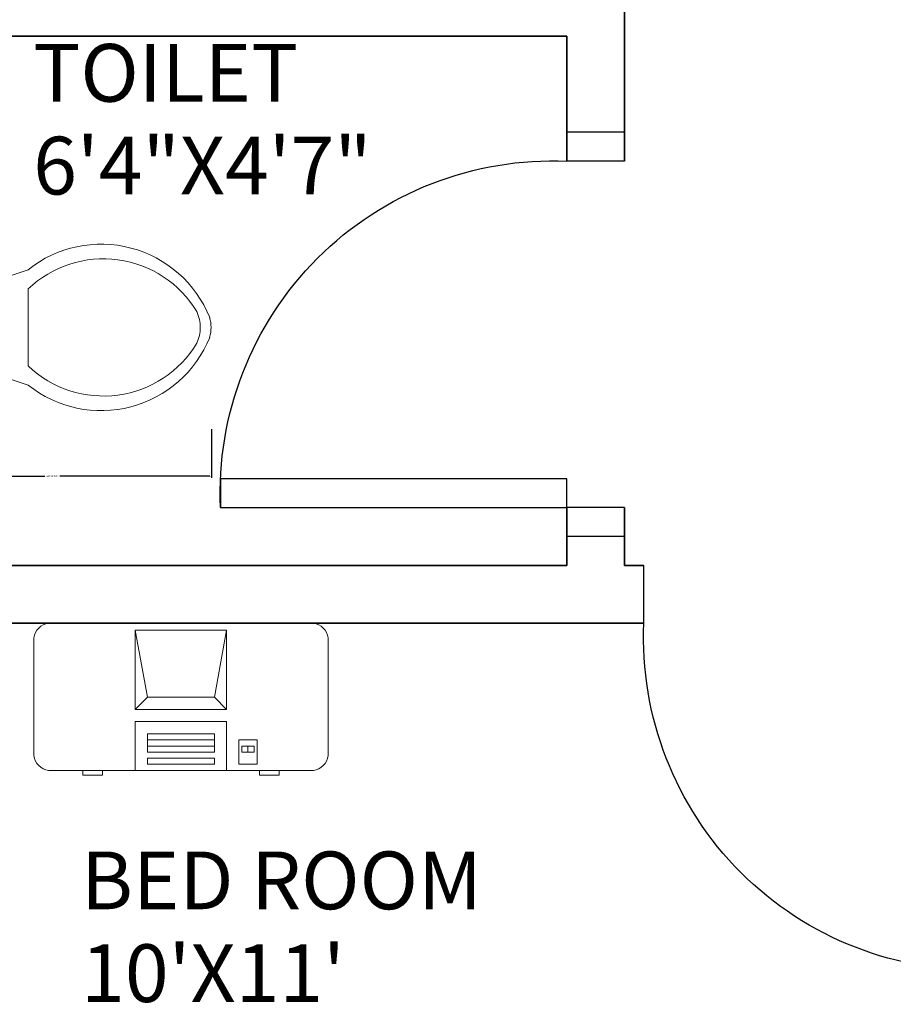
# Model space of a CAD drawing. Units: inches. Extents: x 4159 to 4826, y 299 to 1026.
# Tile 11 of 37: x 4214 to 4305, y 494 to 596. Entities that reach past the tile are written whole.
import ezdxf

# ---------------------------------------------------------------- set-up
doc = ezdxf.new("R2010")
doc.units = ezdxf.units.IN
for name, color, linetype, lineweight in [('A-ANNO-DIMS', 2, 'Continuous', 18), ('A-AREA-IDEN', 7, 'Continuous', 18), ('A-DOOR', 4, 'Continuous', 25), ('A-EQPM', 8, 'Continuous', 13), ('A-FLOR-FIXT', 9, 'Continuous', 18), ('A-FURN', 8, 'Continuous', 18), ('A-WALL', 7, 'Continuous', 35)]:
    doc.layers.add(name, color=color, linetype=linetype, lineweight=lineweight)
doc.styles.get("Standard").update_dxf_attribs({"font": 'arial.ttf'})
doc.dimstyles.get("Standard").update_dxf_attribs({"dimtxt": 0.18, "dimasz": 0.18, "dimexe": 0.18, "dimexo": 0.0625, "dimgap": 0.09, "dimtad": 0, "dimtih": 1, "dimtoh": 1, "dimdec": 4, "dimzin": 0, "dimdsep": 46, "dimtxsty": 'Standard', "dimcen": 0.09, "dimadec": 0, "dimazin": 0, "dimtfac": 1, "dimtdec": 4, "dimtofl": 0, "dimtmove": 0, "dimatfit": 3, "dimfxl": 1, "dimtolj": 1, "dimtzin": 0, "dimarcsym": 0})

# ---------------------------------------------------------------- blocks, each defined once
blk = doc.blocks.new('Toilet - top')
for p, q in [((9.5, -6), (9.5, -2)), ((-8, -8.5), (-8, -8)), ((-7, -8), (-7, -9.5)), ((-4, -8), (-6, -14)), ((4, -8), (6, -14)), ((-10, -8.5), (-8, -8.5)), ((-10, -9.5), (-10, -8.5)), ((-7, -9.5), (-10, -9.5)), ((4, -14), (-4, -14))]:
    blk.add_line(p, q)
blk.add_lwpolyline([(10.5, -8), (10.5, 0), (-10.5, 0), (-10.5, -8)], close=True)
for points in [[(8.5, -1), (-8.5, -1)], [(-9.5, -2), (-9.5, -6)], [(-8.5, -7), (8.5, -7)]]:
    blk.add_lwpolyline(points)
for centre, radius, start, end in [((-8.62, -1.88), 0.884, 81.8699, 188.1301), ((8.62, -1.88), 0.884, 351.8699, 98.1301), ((-8.62, -6.12), 0.884, 171.8699, 278.1301), ((8.62, -6.12), 0.884, 261.8699, 8.1301), ((3.52, -21.58), 12.17, 141.4691, 247.9714), ((4.2, -21.82), 11.33, 136.3677, 238.9468), ((-3.52, -21.58), 12.17, 292.0284, 38.5307), ((-4.2, -21.82), 11.33, 301.053, 43.6321), ((0, -27.88), 4, 245.7318, 294.2682), ((0, -29), 4, 254.8605, 285.1395)]:
    blk.add_arc(centre, radius, start, end)
blk = doc.blocks.new('Desk - 30 x 60 in.')
for p, q in [((-26.999995, 0), (26.999995, 0)), ((-29.999995, -27), (-29.999995, -3)), ((29.999995, -3), (29.999995, -27)), ((26.999995, -30), (-26.999995, -30)), ((-20.000005, -30), (-20.000005, -31)), ((-16.000005, -31), (-16.000005, -30)), ((15.999995, -31), (15.999995, -30)), ((19.999995, -30), (19.999995, -31)), ((-20.000005, -31), (-16.000005, -31)), ((19.999995, -31), (15.999995, -31))]:
    blk.add_line(p, q)
for centre, start, end in [((-26.499995, -3.5), 98.1301, 171.8699), ((26.499995, -3.5), 8.130102, 81.8699), ((-26.499995, -26.5), 188.1301, 261.8699), ((26.499995, -26.5), 278.1301, 351.8699)]:
    blk.add_arc(centre, 3.535534, start, end)
blk = doc.blocks.new('Computer Terminal')
for p, q in [((-10, 11.5), (5, 11.5)), ((-8, 0.5), (-10, 11.5)), ((-10, -1.5), (-10, 11.5)), ((5, 11.5), (3, 0.5)), ((5, 11.5), (5, -1.5)), ((-10, -1.5), (-8, 0.5)), ((3, 0.5), (-8, 0.5)), ((3, 0.5), (5, -1.5)), ((5, -1.5), (-10, -1.5)), ((-10, -11.5), (-10, -3.5)), ((-10, -3.5), (5, -3.5)), ((5, -3.5), (5, -11.5)), ((-8, -5.5), (-8, -8.5)), ((3, -5.5), (-8, -5.5)), ((3, -8.5), (3, -5.5)), ((3, -6.5), (-8, -6.5)), ((-8, -7.5), (3, -7.5)), ((10, -6.5), (7, -6.5)), ((7, -6.5), (7, -10.5)), ((9.5, -7.5), (7.5, -7.5)), ((7.5, -7.5), (7.5, -8.5)), ((8.5, -7.5), (8.5, -8.5)), ((9.5, -8.5), (9.5, -7.5)), ((10, -10.5), (10, -6.5)), ((-8, -8.5), (3, -8.5)), ((-8, -9.5), (-8, -10.5)), ((3, -9.5), (-8, -9.5)), ((3, -10.5), (3, -9.5)), ((7.5, -8.5), (9.5, -8.5)), ((-8, -10.5), (3, -10.5)), ((7, -10.5), (10, -10.5)), ((5, -11.5), (-10, -11.5))]:
    blk.add_line(p, q)
blk = doc.blocks.new('DOOR-SWING-36IN')
blk.add_lwpolyline([(0, 0), (-3, 0), (-3, 36), (0, 36)], close=True)
blk.add_arc((-1.5, 1.5), 34.53, 87.5104, 182.4896)
blk = doc.blocks.new('DOOR-FRAME-36IN')
for p, q in [((0, 6), (0, 0)), ((3, 6), (3, 0)), ((39, 6), (39, 0)), ((42, 6), (42, 0))]:
    blk.add_line(p, q)
blk = doc.blocks.new('*D37')
at = {"layer": 'A-ANNO-DIMS', "color": 0, "lineweight": -2, "transparency": 16777216}
for p, q in [((4201.32, 553.41), (4201.32, 548.34)), ((4234.37, 553.41), (4234.37, 548.34)), ((4201.5, 548.52), (4217.07, 548.52)), ((4234.19, 548.52), (4218.62, 548.52))]:
    blk.add_line(p, q, dxfattribs=at)
at = {"layer": 'A-ANNO-DIMS', "color": 0, "transparency": 16777216}
for points in [[(4201.5, 548.55), (4201.5, 548.49), (4201.32, 548.52)], [(4234.19, 548.55), (4234.19, 548.49), (4234.37, 548.52)]]:
    blk.add_solid(points, dxfattribs=at)
at = {"layer": 'Defpoints', "color": 0, "transparency": 16777216}
for p in [(4201.32, 553.48), (4234.37, 553.48), (4201.32, 548.52)]:
    blk.add_point(p, dxfattribs=at)
at = {"layer": 'A-ANNO-DIMS', "color": 0, "transparency": 16777216, "insert": (4217.85, 548.52), "char_height": 0.18, "attachment_point": 5}
blk.add_mtext('\\A1;WC 33 TYP.', dxfattribs=at)
blk = doc.blocks.new('*D44')
at = {"layer": 'A-ANNO-DIMS', "color": 0, "lineweight": -2, "transparency": 16777216}
for p, q in [((4287.26, 963.09), (4158.88, 963.09)), ((4159.06, 962.91), (4159.06, 647.83)), ((4159.06, 332.38), (4159.06, 647.46)), ((4447.25, 332.2), (4158.88, 332.2))]:
    blk.add_line(p, q, dxfattribs=at)
at = {"layer": 'A-ANNO-DIMS', "color": 0, "transparency": 16777216}
for points in [[(4159.03, 962.91), (4159.09, 962.91), (4159.06, 963.09)], [(4159.03, 332.38), (4159.09, 332.38), (4159.06, 332.2)]]:
    blk.add_solid(points, dxfattribs=at)
at = {"layer": 'Defpoints', "color": 0, "transparency": 16777216}
for p in [(4287.33, 963.09), (4159.06, 332.2), (4447.31, 332.2)]:
    blk.add_point(p, dxfattribs=at)
at = {"layer": 'A-ANNO-DIMS', "color": 0, "transparency": 16777216, "insert": (4159.06, 647.64), "char_height": 0.18, "attachment_point": 5}
blk.add_mtext('\\A1;630.9', dxfattribs=at)

msp = doc.modelspace()

# ---------------------------------------------------------------- linework, layer by layer
at = {"layer": 'A-DOOR'}
msp.add_line((4279.31, 533.254), (4279.31, 539.254), dxfattribs=at)
at = {"layer": 'A-WALL'}
for p, q in [((4277.31, 594.254), (4277.31, 600.254)), ((4271.31, 594.254), (4201.31, 594.254)), ((4271.31, 594.254), (4271.31, 581.254)), ((4277.31, 594.254), (4277.31, 581.254)), ((4271.31, 545.254), (4271.31, 539.254)), ((4277.31, 545.254), (4277.31, 539.254)), ((4271.31, 539.254), (4201.31, 539.254)), ((4279.31, 539.254), (4277.31, 539.254)), ((4279.31, 533.254), (4201.31, 533.254))]:
    msp.add_line(p, q, dxfattribs=at)

# ---------------------------------------------------------------- block references
at = {"layer": 'A-DOOR', "rotation": 270.0000000000003}
msp.add_blockref('DOOR-FRAME-36IN', (4271.31, 584.254), dxfattribs=at)
at = {"layer": 'A-DOOR', "extrusion": (0, 0, -1), "zscale": -1}
for p, rotation in [((-4271.31, 545.254), 270.0000000000011), ((-4315.31, 533.254), 180)]:
    msp.add_blockref('DOOR-SWING-36IN', p, dxfattribs=dict(at, rotation=rotation))
at = {"layer": 'A-EQPM', "xscale": 0.6328414688201627, "yscale": 0.6328414688201627, "zscale": 0.6328414688201627}
msp.add_blockref('Computer Terminal', (4232.783, 525.235), dxfattribs=at)
at = {"layer": 'A-FLOR-FIXT', "rotation": 90}
msp.add_blockref('Toilet - top', (4201.323, 563.977), dxfattribs=at)
at = {"layer": 'A-FURN', "xscale": 0.5098837128326598, "yscale": 0.5098837128326598, "zscale": 0.5098837128326598}
msp.add_blockref('Desk - 30 x 60 in.', (4231.201, 533.254), dxfattribs=at)

# ---------------------------------------------------------------- texts
at = {"layer": 'A-AREA-IDEN'}
for s, p in [('TOILET', (4215.847, 587.428)), ('6\'4"X4\'7"', (4215.847, 577.789)), ('BED ROOM', (4220.833, 503.526)), ("10'X11'", (4220.833, 493.887))]:
    msp.add_text(s, height=6, dxfattribs=at).set_placement(p)

# ---------------------------------------------------------------- dimensions: what is measured, and where the dimension line sits
at = {"layer": 'A-ANNO-DIMS'}
dim = msp.add_linear_dim(base=(4159.06, 332.195), p1=(4287.326, 963.093), p2=(4447.31, 332.195), angle=90, dimstyle='Standard', override={"dimdec": 1, "dimlfac": 1, "dimrnd": 0, "dimzin": 0, "dimdsep": 46, "dimlunit": 2}, dxfattribs=at)
dim.commit()
dim.dimension.update_dxf_attribs({"geometry": '*D44', "text_midpoint": (4159.06, 647.644)})
dim = msp.add_linear_dim(base=(4201.323, 548.52), p1=(4234.369, 553.477), p2=(4201.323, 553.477), angle=180, text='WC <> TYP.', dimstyle='Standard', override={"dimdec": 0, "dimlfac": 1, "dimrnd": 0, "dimzin": 0, "dimdsep": 46, "dimlunit": 2}, dxfattribs=at)
dim.commit()
dim.dimension.update_dxf_attribs({"geometry": '*D37', "text_midpoint": (4217.846, 548.52)})

doc.saveas('drawing.dxf')
